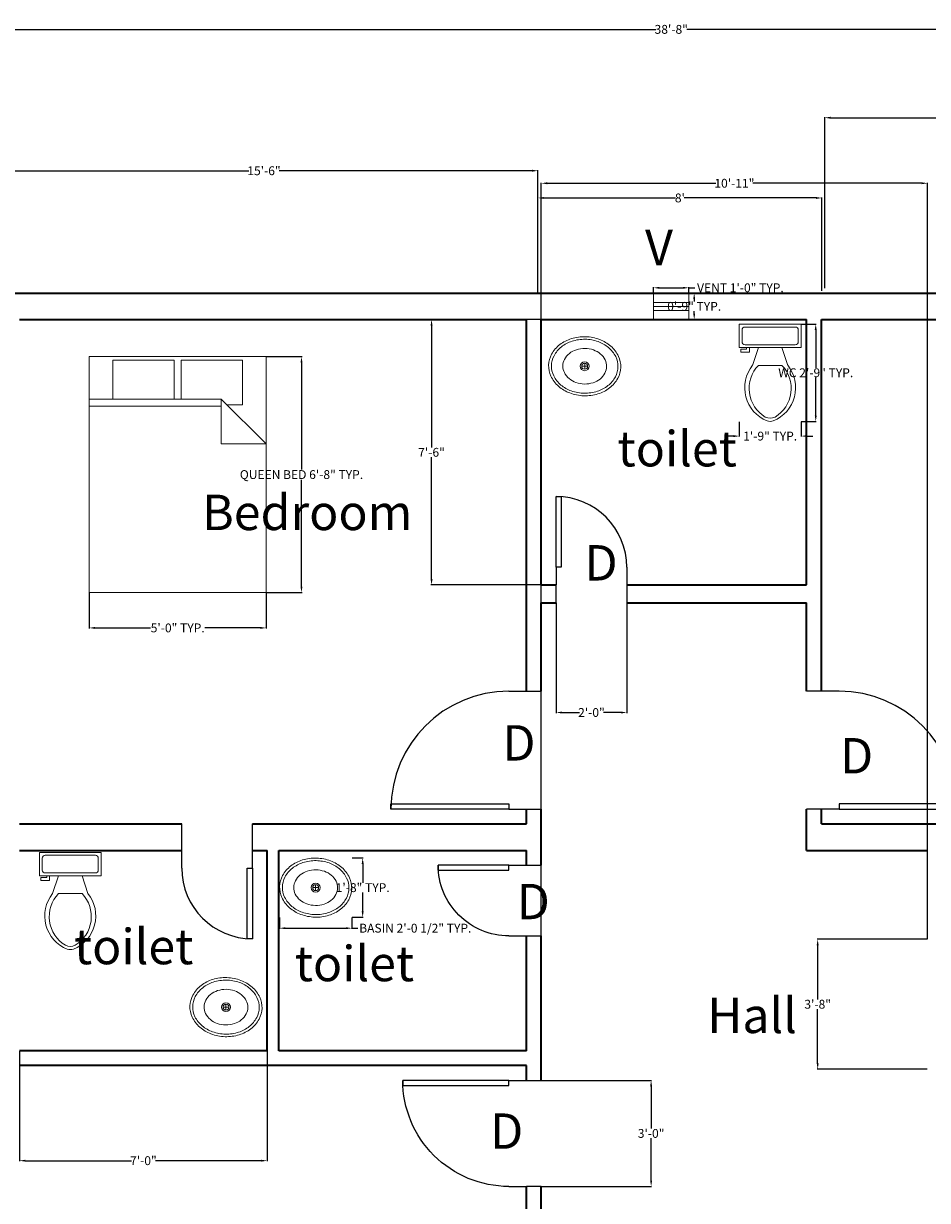
# Model space of a CAD drawing. Units: inches. Extents: x 751 to 1500, y 610 to 1297.
# Tile 3 of 4: x 1001 to 1308, y 898 to 1297. Entities that reach past the tile are written whole.
import ezdxf

# ---------------------------------------------------------------- set-up
doc = ezdxf.new("R2010")
doc.units = ezdxf.units.IN
doc.header["$MEASUREMENT"] = 0
doc.layers.get('0').update_dxf_attribs({"color": 1})
for name, color, linetype, lineweight in [('A-ANNO-DIMS', 5, 'Continuous', 18), ('A-ANNO-TEXT', 7, 'Continuous', 18), ('A-AREA-IDEN', 7, 'Continuous', 25), ('A-FLOR-FIXT', 9, 'Continuous', 18), ('A-FURN', 8, 'Continuous', 18), ('door', 2, 'Continuous', 25), ('wall', 6, 'Continuous', 35), ('windows', 70, 'Continuous', 18)]:
    doc.layers.add(name, color=color, linetype=linetype, lineweight=lineweight)
doc.styles.get("Standard").update_dxf_attribs({"font": 'arial.ttf'})
doc.dimstyles.get("Standard").update_dxf_attribs({"dimtxt": 3, "dimasz": 2, "dimexe": 0.18, "dimexo": 0.0625, "dimgap": 0.09, "dimtad": 0, "dimtih": 1, "dimtoh": 1, "dimdec": 0, "dimzin": 0, "dimdsep": 46, "dimlunit": 3, "dimtxsty": 'Standard', "dimcen": 0.09, "dimadec": 0, "dimazin": 0, "dimtfac": 1, "dimtdec": 0, "dimtofl": 0, "dimtmove": 0, "dimatfit": 3, "dimfxl": 1, "dimtolj": 1, "dimtzin": 0, "dimarcsym": 0})

# ---------------------------------------------------------------- blocks, each defined once
blk = doc.blocks.new('*U2')
for p, q in [((0, 0), (0, -6)), ((40, 0), (40, -6))]:
    blk.add_line(p, q)
blk.add_lwpolyline([(0, 0), (0, 40), (1.75, 40), (1.75, 0)], close=True)
blk.add_arc((0, 0), 40, 0, 90)
blk = doc.blocks.new('*U3')
for p, q in [((0, 0), (0, 6)), ((40, 0), (40, 6))]:
    blk.add_line(p, q)
blk.add_lwpolyline([(0, 0), (0, -40), (1.75, -40), (1.75, 0)], close=True)
blk.add_arc((0, 0), 40, 270, 360)
blk = doc.blocks.new('*U4')
for p, q in [((0, 0), (0, -6)), ((24, 0), (24, -6))]:
    blk.add_line(p, q)
blk.add_lwpolyline([(0, 0), (0, 24), (1.75, 24), (1.75, 0)], close=True)
blk.add_arc((0, 0), 24, 0, 90)
blk = doc.blocks.new('*U7')
for p, q in [((0, 0), (0, -6)), ((36, 0), (36, -6))]:
    blk.add_line(p, q)
blk.add_lwpolyline([(0, 0), (0, 36), (1.75, 36), (1.75, 0)], close=True)
blk.add_arc((0, 0), 36, 0, 90)
blk = doc.blocks.new('*D8')
at = {"layer": 'A-ANNO-DIMS', "color": 0, "lineweight": -2, "transparency": 16777216}
for p, q in [((989.16, 1207.18), (989.16, 1295.32)), ((991.16, 1295.14), (1215.8, 1295.14)), ((1450.93, 1295.14), (1226.29, 1295.14)), ((1452.93, 1205.96), (1452.93, 1295.32))]:
    blk.add_line(p, q, dxfattribs=at)
at = {"layer": 'A-ANNO-DIMS', "color": 0, "transparency": 16777216}
for points in [[(991.16, 1295.48), (991.16, 1294.81), (989.16, 1295.14)], [(1450.93, 1295.48), (1450.93, 1294.81), (1452.93, 1295.14)]]:
    blk.add_solid(points, dxfattribs=at)
at = {"layer": 'Defpoints', "color": 0, "transparency": 16777216}
for p in [(1452.93, 1295.14), (989.16, 1207.12), (1452.93, 1205.9)]:
    blk.add_point(p, dxfattribs=at)
at = {"layer": 'A-ANNO-DIMS', "color": 0, "transparency": 16777216, "insert": (1221.05, 1295.14), "char_height": 3, "attachment_point": 5}
blk.add_mtext('\\A1;38\'-8"', dxfattribs=at)
blk = doc.blocks.new('*D9')
at = {"layer": 'A-ANNO-DIMS', "color": 0, "lineweight": -2, "transparency": 16777216}
for p, q in [((989.97, 1205.95), (989.97, 1247.37)), ((991.97, 1247.19), (1077.79, 1247.19)), ((1173.82, 1247.19), (1088, 1247.19)), ((1175.82, 1205.95), (1175.82, 1247.37))]:
    blk.add_line(p, q, dxfattribs=at)
at = {"layer": 'A-ANNO-DIMS', "color": 0, "transparency": 16777216}
for points in [[(991.97, 1247.53), (991.97, 1246.86), (989.97, 1247.19)], [(1173.82, 1247.53), (1173.82, 1246.86), (1175.82, 1247.19)]]:
    blk.add_solid(points, dxfattribs=at)
at = {"layer": 'Defpoints', "color": 0, "transparency": 16777216}
for p in [(1175.82, 1247.19), (989.97, 1205.88), (1175.82, 1205.88)]:
    blk.add_point(p, dxfattribs=at)
at = {"layer": 'A-ANNO-DIMS', "color": 0, "transparency": 16777216, "insert": (1082.89, 1247.19), "char_height": 3, "attachment_point": 5}
blk.add_mtext('\\A1;15\'-6"', dxfattribs=at)
blk = doc.blocks.new('*D10')
at = {"layer": 'A-ANNO-DIMS', "color": 0, "lineweight": -2, "transparency": 16777216}
for p, q in [((1175.82, 1206.43), (1175.82, 1238.14)), ((1177.82, 1237.96), (1222.52, 1237.96)), ((1270.16, 1237.96), (1225.46, 1237.96)), ((1272.16, 1206.43), (1272.16, 1238.14))]:
    blk.add_line(p, q, dxfattribs=at)
at = {"layer": 'A-ANNO-DIMS', "color": 0, "transparency": 16777216}
for points in [[(1177.82, 1238.29), (1177.82, 1237.63), (1175.82, 1237.96)], [(1270.16, 1238.29), (1270.16, 1237.63), (1272.16, 1237.96)]]:
    blk.add_solid(points, dxfattribs=at)
at = {"layer": 'Defpoints', "color": 0, "transparency": 16777216}
for p in [(1272.16, 1237.96), (1175.82, 1206.37), (1272.16, 1206.37)]:
    blk.add_point(p, dxfattribs=at)
at = {"layer": 'A-ANNO-DIMS', "color": 0, "transparency": 16777216, "insert": (1223.99, 1237.96), "char_height": 3, "attachment_point": 5}
blk.add_mtext("\\A1;8'", dxfattribs=at)
blk = doc.blocks.new('*D11')
at = {"layer": 'A-ANNO-DIMS', "color": 0, "lineweight": -2, "transparency": 16777216}
for p, q in [((1273.13, 1207.41), (1273.13, 1265.35)), ((1452.66, 1205.46), (1452.66, 1265.35)), ((1275.13, 1265.17), (1360.4, 1265.17)), ((1450.66, 1265.17), (1365.39, 1265.17))]:
    blk.add_line(p, q, dxfattribs=at)
at = {"layer": 'A-ANNO-DIMS', "color": 0, "transparency": 16777216}
for points in [[(1275.13, 1265.51), (1275.13, 1264.84), (1273.13, 1265.17)], [(1450.66, 1265.51), (1450.66, 1264.84), (1452.66, 1265.17)]]:
    blk.add_solid(points, dxfattribs=at)
at = {"layer": 'Defpoints', "color": 0, "transparency": 16777216}
for p in [(1452.66, 1265.17), (1273.13, 1207.34), (1452.66, 1205.4)]:
    blk.add_point(p, dxfattribs=at)
at = {"layer": 'A-ANNO-DIMS', "color": 0, "transparency": 16777216, "insert": (1362.9, 1265.17), "char_height": 3, "attachment_point": 5}
blk.add_mtext("\\A1;15'", dxfattribs=at)
blk = doc.blocks.new('Bed - Queen')
for p, q in [((0, -80.00003), (0, 0)), ((0, 0), (59.99999, 0)), ((59.99999, 0), (59.99999, -80.00003)), ((7.99999, -1.2), (28.79998, -1.2)), ((7.99999, -14.4), (7.99999, -1.2)), ((28.79998, -1.2), (28.79998, -14.4)), ((31.19999, -1.2), (51.99999, -1.2)), ((31.19999, -14.4), (31.19999, -1.2)), ((51.99999, -1.2), (51.99999, -16.4)), ((0, -14.4), (44.8, -14.4)), ((59.99999, -29.6), (44.8, -14.4)), ((44.8, -14.4), (44.8, -29.6)), ((44.8, -16.8), (0, -16.8)), ((51.99999, -16.4), (46.79936, -16.4)), ((44.8, -29.6), (59.99999, -29.6)), ((59.99999, -80.00003), (0, -80.00003))]:
    blk.add_line(p, q)
blk = doc.blocks.new('Sink - Oval top')
for p, q in [((-1, 0), (1, 0)), ((0, 1), (0, -1))]:
    blk.add_line(p, q)
for points in [[(-12.23, 0.39, 0.117634), (-11.46, -3.36, 0.104469), (-8.88, -6.8, 0.090016), (-5.08, -9.07, 0.08192), (-0.32, -10.02, 0.08192), (4.49, -9.38, 0.090016), (8.42, -7.36, 0.104469), (11.22, -4.09, 0.117634), (12.23, -0.39, 0.117634), (11.46, 3.36, 0.104469), (8.88, 6.8, 0.090016), (5.08, 9.07, 0.08192), (0.32, 10.02, 0.08192), (-4.49, 9.38, 0.090016), (-8.42, 7.36, 0.104469), (-11.22, 4.09, 0.117634)], [(-11.29, 0.16, 0.118622), (-10.52, -3.25, 0.104678), (-8.07, -6.36, 0.089562), (-4.54, -8.37, 0.081185), (-0.13, -9.15, 0.081185), (4.3, -8.49, 0.089562), (7.89, -6.58, 0.104678), (10.42, -3.55, 0.118622), (11.29, -0.16, 0.118622), (10.52, 3.25, 0.104678), (8.07, 6.36, 0.089562), (4.54, 8.37, 0.081185), (0.13, 9.15, 0.081185), (-4.3, 8.49, 0.089562), (-7.89, 6.58, 0.104678), (-10.42, 3.55, 0.118622)], [(-7.42, 0.08, 0.118283), (-6.91, -2.17, 0.104607), (-5.29, -4.21, 0.089718), (-2.97, -5.53, 0.081436), (-0.07, -6.04, 0.081436), (2.84, -5.59, 0.089718), (5.2, -4.33, 0.104607), (6.86, -2.32, 0.118283), (7.42, -0.08, 0.118283), (6.91, 2.17, 0.104607), (5.29, 4.21, 0.089718), (2.97, 5.53, 0.081436), (0.07, 6.04, 0.081436), (-2.84, 5.59, 0.089718), (-5.2, 4.33, 0.104607), (-6.86, 2.32, 0.118283)]]:
    blk.add_lwpolyline(points, format="xyb", close=True)
for radius in [1.5, 1]:
    blk.add_circle((0, 0), radius)
blk = doc.blocks.new('Toilet - top')
for p, q in [((9.5, -6), (9.5, -2)), ((-10, -8.5), (-8, -8.5)), ((-10, -9.5), (-10, -8.5)), ((-7, -9.5), (-10, -9.5)), ((-8, -8.5), (-8, -8)), ((-7, -8), (-7, -9.5)), ((-4, -8), (-6, -14)), ((4, -8), (6, -14)), ((4, -14), (-4, -14))]:
    blk.add_line(p, q)
blk.add_lwpolyline([(10.5, -8), (10.5, 0), (-10.5, 0), (-10.5, -8)], close=True)
for points in [[(-9.5, -2), (-9.5, -6)], [(8.5, -1), (-8.5, -1)], [(-8.5, -7), (8.5, -7)]]:
    blk.add_lwpolyline(points)
for centre, radius, start, end in [((-8.62, -1.88), 0.884, 81.8699, 188.1301), ((8.62, -1.88), 0.884, 351.8699, 98.1301), ((-8.62, -6.12), 0.884, 171.8699, 278.1301), ((8.62, -6.12), 0.884, 261.8699, 8.1301), ((3.52, -21.58), 12.17, 141.4691, 247.9714), ((4.2, -21.82), 11.33, 136.3677, 238.9468), ((-3.52, -21.58), 12.17, 292.0284, 38.5307), ((-4.2, -21.82), 11.33, 301.053, 43.6321), ((0, -27.88), 4, 245.7318, 294.2682), ((0, -29), 4, 254.8605, 285.1395)]:
    blk.add_arc(centre, radius, start, end)
blk = doc.blocks.new('VENT-12IN-PLAN')
for p, q in [((3.14, 12), (3.14, 0)), ((4.5, 12), (4.5, 0)), ((5.86, 12), (5.86, 0))]:
    blk.add_line(p, q)
blk.add_lwpolyline([(0, 0), (9, 0), (9, 12), (0, 12)], close=True)
blk = doc.blocks.new('*D31')
at = {"layer": 'A-ANNO-DIMS', "color": 0, "lineweight": -2, "transparency": 16777216}
for p, q in [((1215.04, 1205.75), (1215.04, 1207.67)), ((1217.04, 1207.49), (1225.04, 1207.49)), ((1227.04, 1205.75), (1227.04, 1207.67)), ((1227.04, 1207.49), (1229.04, 1207.49))]:
    blk.add_line(p, q, dxfattribs=at)
at = {"layer": 'A-ANNO-DIMS', "color": 0, "transparency": 16777216}
for points in [[(1217.04, 1207.82), (1217.04, 1207.16), (1215.04, 1207.49)], [(1225.04, 1207.82), (1225.04, 1207.16), (1227.04, 1207.49)]]:
    blk.add_solid(points, dxfattribs=at)
at = {"layer": 'Defpoints', "color": 0, "transparency": 16777216}
for p in [(1215.04, 1205.69), (1227.04, 1207.49), (1227.04, 1205.69)]:
    blk.add_point(p, dxfattribs=at)
at = {"layer": 'A-ANNO-DIMS', "color": 0, "transparency": 16777216, "insert": (1244.52, 1207.49), "char_height": 3, "attachment_point": 5}
blk.add_mtext('\\A1;VENT 1\'-0" TYP.', dxfattribs=at)
blk = doc.blocks.new('*D32')
at = {"layer": 'A-ANNO-DIMS', "color": 0, "lineweight": -2, "transparency": 16777216}
for p, q in [((1227.1, 1205.69), (1229.02, 1205.69)), ((1228.84, 1203.69), (1228.84, 1202.81)), ((1228.84, 1198.69), (1228.84, 1199.57)), ((1227.1, 1196.69), (1229.02, 1196.69))]:
    blk.add_line(p, q, dxfattribs=at)
at = {"layer": 'A-ANNO-DIMS', "color": 0, "transparency": 16777216}
for points in [[(1228.51, 1203.69), (1229.17, 1203.69), (1228.84, 1205.69)], [(1228.51, 1198.69), (1229.17, 1198.69), (1228.84, 1196.69)]]:
    blk.add_solid(points, dxfattribs=at)
at = {"layer": 'Defpoints', "color": 0, "transparency": 16777216}
for p in [(1227.04, 1205.69), (1227.04, 1196.69), (1228.84, 1196.69)]:
    blk.add_point(p, dxfattribs=at)
at = {"layer": 'A-ANNO-DIMS', "color": 0, "transparency": 16777216, "insert": (1228.84, 1201.19), "char_height": 3, "attachment_point": 5}
blk.add_mtext('\\A1;0\'-9" TYP.', dxfattribs=at)
blk = doc.blocks.new('*D33')
at = {"layer": 'A-ANNO-DIMS', "color": 0, "lineweight": -2, "transparency": 16777216}
for p, q in [((1083.67, 1184.14), (1095.79, 1184.14)), ((1095.61, 1182.14), (1095.61, 1145.87)), ((1095.61, 1106.14), (1095.61, 1142.4)), ((1083.67, 1104.14), (1095.79, 1104.14))]:
    blk.add_line(p, q, dxfattribs=at)
at = {"layer": 'A-ANNO-DIMS', "color": 0, "transparency": 16777216}
for points in [[(1095.28, 1182.14), (1095.95, 1182.14), (1095.61, 1184.14)], [(1095.28, 1106.14), (1095.95, 1106.14), (1095.61, 1104.14)]]:
    blk.add_solid(points, dxfattribs=at)
at = {"layer": 'Defpoints', "color": 0, "transparency": 16777216}
for p in [(1083.61, 1184.14), (1095.61, 1184.14), (1083.61, 1104.14)]:
    blk.add_point(p, dxfattribs=at)
at = {"layer": 'A-ANNO-DIMS', "color": 0, "transparency": 16777216, "insert": (1095.61, 1144.14), "char_height": 3, "attachment_point": 5}
blk.add_mtext('\\A1;QUEEN BED 6\'-8" TYP.', dxfattribs=at)
blk = doc.blocks.new('*D34')
at = {"layer": 'A-ANNO-DIMS', "color": 0, "lineweight": -2, "transparency": 16777216}
for p, q in [((1023.61, 1104.07), (1023.61, 1091.96)), ((1083.61, 1104.07), (1083.61, 1091.96)), ((1025.61, 1092.14), (1044.38, 1092.14)), ((1081.61, 1092.14), (1062.85, 1092.14))]:
    blk.add_line(p, q, dxfattribs=at)
at = {"layer": 'A-ANNO-DIMS', "color": 0, "transparency": 16777216}
for points in [[(1025.61, 1092.47), (1025.61, 1091.8), (1023.61, 1092.14)], [(1081.61, 1092.47), (1081.61, 1091.8), (1083.61, 1092.14)]]:
    blk.add_solid(points, dxfattribs=at)
at = {"layer": 'Defpoints', "color": 0, "transparency": 16777216}
for p in [(1023.61, 1104.14), (1083.61, 1104.14), (1083.61, 1092.14)]:
    blk.add_point(p, dxfattribs=at)
at = {"layer": 'A-ANNO-DIMS', "color": 0, "transparency": 16777216, "insert": (1053.61, 1092.14), "char_height": 3, "attachment_point": 5}
blk.add_mtext('\\A1;5\'-0" TYP.', dxfattribs=at)
blk = doc.blocks.new('*D35')
at = {"layer": 'A-ANNO-DIMS', "color": 0, "lineweight": -2, "transparency": 16777216}
for p, q in [((1088.14, 993.92), (1088.14, 990.12)), ((1112.69, 993.92), (1112.69, 990.12)), ((1090.14, 990.3), (1110.69, 990.3)), ((1112.69, 990.3), (1114.69, 990.3))]:
    blk.add_line(p, q, dxfattribs=at)
at = {"layer": 'A-ANNO-DIMS', "color": 0, "transparency": 16777216}
for points in [[(1090.14, 990.63), (1090.14, 989.96), (1088.14, 990.3)], [(1110.69, 990.63), (1110.69, 989.96), (1112.69, 990.3)]]:
    blk.add_solid(points, dxfattribs=at)
at = {"layer": 'Defpoints', "color": 0, "transparency": 16777216}
for p in [(1088.14, 993.98), (1112.69, 993.98), (1112.69, 990.3)]:
    blk.add_point(p, dxfattribs=at)
at = {"layer": 'A-ANNO-DIMS', "color": 0, "transparency": 16777216, "insert": (1134.22, 990.3), "char_height": 3, "attachment_point": 5}
blk.add_mtext('\\A1;BASIN 2\'-0 1/2" TYP.', dxfattribs=at)
blk = doc.blocks.new('*D36')
at = {"layer": 'A-ANNO-DIMS', "color": 0, "lineweight": -2, "transparency": 16777216}
for p, q in [((1112.75, 1014.12), (1116.55, 1014.12)), ((1116.37, 1012.12), (1116.37, 1005.67)), ((1116.37, 995.98), (1116.37, 1002.43)), ((1112.75, 993.98), (1116.55, 993.98))]:
    blk.add_line(p, q, dxfattribs=at)
at = {"layer": 'A-ANNO-DIMS', "color": 0, "transparency": 16777216}
for points in [[(1116.04, 1012.12), (1116.71, 1012.12), (1116.37, 1014.12)], [(1116.04, 995.98), (1116.71, 995.98), (1116.37, 993.98)]]:
    blk.add_solid(points, dxfattribs=at)
at = {"layer": 'Defpoints', "color": 0, "transparency": 16777216}
for p in [(1112.69, 1014.12), (1116.37, 1014.12), (1112.69, 993.98)]:
    blk.add_point(p, dxfattribs=at)
at = {"layer": 'A-ANNO-DIMS', "color": 0, "transparency": 16777216, "insert": (1116.37, 1004.05), "char_height": 3, "attachment_point": 5}
blk.add_mtext('\\A1;1\'-8" TYP.', dxfattribs=at)
blk = doc.blocks.new('*D37')
at = {"layer": 'A-ANNO-DIMS', "color": 0, "lineweight": -2, "transparency": 16777216}
for p, q in [((1265.18, 1195.19), (1270.26, 1195.19)), ((1270.08, 1193.19), (1270.08, 1180.31)), ((1270.08, 1164.14), (1270.08, 1177.03)), ((1265.18, 1162.14), (1270.26, 1162.14))]:
    blk.add_line(p, q, dxfattribs=at)
at = {"layer": 'A-ANNO-DIMS', "color": 0, "transparency": 16777216}
for points in [[(1269.74, 1193.19), (1270.41, 1193.19), (1270.08, 1195.19)], [(1269.74, 1164.14), (1270.41, 1164.14), (1270.08, 1162.14)]]:
    blk.add_solid(points, dxfattribs=at)
at = {"layer": 'Defpoints', "color": 0, "transparency": 16777216}
for p in [(1265.12, 1195.19), (1270.08, 1195.19), (1265.12, 1162.14)]:
    blk.add_point(p, dxfattribs=at)
at = {"layer": 'A-ANNO-DIMS', "color": 0, "transparency": 16777216, "insert": (1270.08, 1178.67), "char_height": 3, "attachment_point": 5}
blk.add_mtext('\\A1;WC 2\'-9" TYP.', dxfattribs=at)
blk = doc.blocks.new('*D38')
at = {"layer": 'A-ANNO-DIMS', "color": 0, "lineweight": -2, "transparency": 16777216}
for p, q in [((1244.12, 1162.08), (1244.12, 1157.01)), ((1265.12, 1162.08), (1265.12, 1157.01)), ((1242.12, 1157.19), (1240.12, 1157.19)), ((1267.12, 1157.19), (1269.12, 1157.19))]:
    blk.add_line(p, q, dxfattribs=at)
at = {"layer": 'A-ANNO-DIMS', "color": 0, "transparency": 16777216}
for points in [[(1242.12, 1157.52), (1242.12, 1156.85), (1244.12, 1157.19)], [(1267.12, 1157.52), (1267.12, 1156.85), (1265.12, 1157.19)]]:
    blk.add_solid(points, dxfattribs=at)
at = {"layer": 'Defpoints', "color": 0, "transparency": 16777216}
for p in [(1244.12, 1162.14), (1265.12, 1162.14), (1265.12, 1157.19)]:
    blk.add_point(p, dxfattribs=at)
at = {"layer": 'A-ANNO-DIMS', "color": 0, "transparency": 16777216, "insert": (1254.62, 1157.19), "char_height": 3, "attachment_point": 5}
blk.add_mtext('\\A1;1\'-9" TYP.', dxfattribs=at)
blk = doc.blocks.new('*D54')
at = {"layer": 'A-ANNO-DIMS', "color": 0, "lineweight": -2, "transparency": 16777216}
for p, q in [((999.98, 948.63), (999.98, 911.26)), ((1083.98, 948.63), (1083.98, 911.26)), ((1001.98, 911.44), (1037.92, 911.44)), ((1081.98, 911.44), (1046.05, 911.44))]:
    blk.add_line(p, q, dxfattribs=at)
at = {"layer": 'A-ANNO-DIMS', "color": 0, "transparency": 16777216}
for points in [[(1001.98, 911.77), (1001.98, 911.11), (999.98, 911.44)], [(1081.98, 911.77), (1081.98, 911.11), (1083.98, 911.44)]]:
    blk.add_solid(points, dxfattribs=at)
at = {"layer": 'Defpoints', "color": 0, "transparency": 16777216}
for p in [(999.98, 948.69), (1083.98, 948.69), (999.98, 911.44)]:
    blk.add_point(p, dxfattribs=at)
at = {"layer": 'A-ANNO-DIMS', "color": 0, "transparency": 16777216, "insert": (1041.98, 911.44), "char_height": 3, "attachment_point": 5}
blk.add_mtext('\\A1;7\'-0"', dxfattribs=at)
blk = doc.blocks.new('*D56')
at = {"layer": 'A-ANNO-DIMS', "color": 0, "lineweight": -2, "transparency": 16777216}
for p, q in [((1176.92, 1196.69), (1139.55, 1196.69)), ((1139.73, 1194.69), (1139.73, 1153.31)), ((1139.73, 1108.69), (1139.73, 1150.07)), ((1176.92, 1106.69), (1139.55, 1106.69))]:
    blk.add_line(p, q, dxfattribs=at)
at = {"layer": 'A-ANNO-DIMS', "color": 0, "transparency": 16777216}
for points in [[(1139.4, 1194.69), (1140.07, 1194.69), (1139.73, 1196.69)], [(1139.4, 1108.69), (1140.07, 1108.69), (1139.73, 1106.69)]]:
    blk.add_solid(points, dxfattribs=at)
at = {"layer": 'Defpoints', "color": 0, "transparency": 16777216}
for p in [(1139.73, 1196.69), (1176.98, 1196.69), (1176.98, 1106.69)]:
    blk.add_point(p, dxfattribs=at)
at = {"layer": 'A-ANNO-DIMS', "color": 0, "transparency": 16777216, "insert": (1139.73, 1151.69), "char_height": 3, "attachment_point": 5}
blk.add_mtext('\\A1;7\'-6"', dxfattribs=at)
blk = doc.blocks.new('*D58')
at = {"layer": 'A-ANNO-DIMS', "color": 0, "lineweight": -2, "transparency": 16777216}
for p, q in [((1177.04, 938.69), (1214.41, 938.69)), ((1214.23, 936.69), (1214.23, 922.31)), ((1214.23, 904.69), (1214.23, 919.07)), ((1177.04, 902.69), (1214.41, 902.69))]:
    blk.add_line(p, q, dxfattribs=at)
at = {"layer": 'A-ANNO-DIMS', "color": 0, "transparency": 16777216}
for points in [[(1213.9, 936.69), (1214.57, 936.69), (1214.23, 938.69)], [(1213.9, 904.69), (1214.57, 904.69), (1214.23, 902.69)]]:
    blk.add_solid(points, dxfattribs=at)
at = {"layer": 'Defpoints', "color": 0, "transparency": 16777216}
for p in [(1176.98, 938.69), (1176.98, 902.69), (1214.23, 902.69)]:
    blk.add_point(p, dxfattribs=at)
at = {"layer": 'A-ANNO-DIMS', "color": 0, "transparency": 16777216, "insert": (1214.23, 920.69), "char_height": 3, "attachment_point": 5}
blk.add_mtext('\\A1;3\'-0"', dxfattribs=at)
blk = doc.blocks.new('*D59')
at = {"layer": 'A-ANNO-DIMS', "color": 0, "lineweight": -2, "transparency": 16777216}
for p, q in [((1181.98, 1100.63), (1181.98, 1063.26)), ((1205.98, 1100.63), (1205.98, 1063.26)), ((1183.98, 1063.44), (1189.88, 1063.44)), ((1203.98, 1063.44), (1198.09, 1063.44))]:
    blk.add_line(p, q, dxfattribs=at)
at = {"layer": 'A-ANNO-DIMS', "color": 0, "transparency": 16777216}
for points in [[(1183.98, 1063.77), (1183.98, 1063.11), (1181.98, 1063.44)], [(1203.98, 1063.77), (1203.98, 1063.11), (1205.98, 1063.44)]]:
    blk.add_solid(points, dxfattribs=at)
at = {"layer": 'Defpoints', "color": 0, "transparency": 16777216}
for p in [(1181.98, 1100.69), (1205.98, 1100.69), (1181.98, 1063.44)]:
    blk.add_point(p, dxfattribs=at)
at = {"layer": 'A-ANNO-DIMS', "color": 0, "transparency": 16777216, "insert": (1193.98, 1063.44), "char_height": 3, "attachment_point": 5}
blk.add_mtext('\\A1;2\'-0"', dxfattribs=at)
blk = doc.blocks.new('*D62')
at = {"layer": 'A-ANNO-DIMS', "color": 0, "lineweight": -2, "transparency": 16777216}
for p, q in [((1176.98, 987.75), (1176.98, 1243.12)), ((1178.98, 1242.94), (1236.22, 1242.94)), ((1305.98, 1242.94), (1248.75, 1242.94)), ((1307.98, 986.59), (1307.98, 1243.12))]:
    blk.add_line(p, q, dxfattribs=at)
at = {"layer": 'A-ANNO-DIMS', "color": 0, "transparency": 16777216}
for points in [[(1178.98, 1243.27), (1178.98, 1242.61), (1176.98, 1242.94)], [(1305.98, 1243.27), (1305.98, 1242.61), (1307.98, 1242.94)]]:
    blk.add_solid(points, dxfattribs=at)
at = {"layer": 'Defpoints', "color": 0, "transparency": 16777216}
for p in [(1307.98, 1242.94), (1176.98, 987.69), (1307.98, 986.52)]:
    blk.add_point(p, dxfattribs=at)
at = {"layer": 'A-ANNO-DIMS', "color": 0, "transparency": 16777216, "insert": (1242.48, 1242.94), "char_height": 3, "attachment_point": 5}
blk.add_mtext('\\A1;10\'-11"', dxfattribs=at)
blk = doc.blocks.new('*D66')
at = {"layer": 'A-ANNO-DIMS', "color": 0, "lineweight": -2, "transparency": 16777216}
for p, q in [((1307.92, 986.52), (1270.55, 986.52)), ((1270.73, 984.52), (1270.73, 966.12)), ((1270.73, 944.48), (1270.73, 962.88)), ((1307.92, 942.48), (1270.55, 942.48))]:
    blk.add_line(p, q, dxfattribs=at)
at = {"layer": 'A-ANNO-DIMS', "color": 0, "transparency": 16777216}
for points in [[(1270.4, 984.52), (1271.07, 984.52), (1270.73, 986.52)], [(1270.4, 944.48), (1271.07, 944.48), (1270.73, 942.48)]]:
    blk.add_solid(points, dxfattribs=at)
at = {"layer": 'Defpoints', "color": 0, "transparency": 16777216}
for p in [(1270.73, 986.52), (1307.98, 986.52), (1307.98, 942.48)]:
    blk.add_point(p, dxfattribs=at)
at = {"layer": 'A-ANNO-DIMS', "color": 0, "transparency": 16777216, "insert": (1270.73, 964.5), "char_height": 3, "attachment_point": 5}
blk.add_mtext('\\A1;3\'-8"', dxfattribs=at)

msp = doc.modelspace()

# ---------------------------------------------------------------- linework, layer by layer
at = {"layer": 'door'}
for p, q in [((1181.98, 1100.69), (1181.98, 1106.69)), ((1205.98, 1106.69), (1205.98, 1100.69)), ((1171.98, 1070.69), (1176.98, 1070.69)), ((1271.98, 1070.69), (1266.98, 1070.69)), ((1171.98, 1030.69), (1176.98, 1030.69)), ((1271.98, 1030.69), (1266.98, 1030.69)), ((1054.98, 1016.69), (1054.98, 1025.69)), ((1078.98, 1016.69), (1078.98, 1025.69)), ((1171.98, 1011.69), (1176.98, 1011.69)), ((1171.98, 987.69), (1176.98, 987.69)), ((1171.98, 938.69), (1176.98, 938.69)), ((1176.98, 902.69), (1171.98, 902.69))]:
    msp.add_line(p, q, dxfattribs=at)
at = {"layer": 'wall'}
for p, q in [((990.98, 1205.69), (1296.98, 1205.69)), ((1296.98, 1205.69), (1453.98, 1205.69)), ((999.98, 1196.69), (1171.98, 1196.69)), ((1171.98, 1070.69), (1171.98, 1196.69)), ((1176.98, 1196.69), (1266.98, 1196.69)), ((1176.98, 1106.69), (1176.98, 1196.69)), ((1266.98, 1106.69), (1266.98, 1196.69)), ((1271.98, 1196.69), (1296.98, 1196.69)), ((1271.98, 1070.69), (1271.98, 1196.69)), ((1296.98, 1196.69), (1444.98, 1196.69)), ((1176.98, 1106.69), (1181.98, 1106.69)), ((1205.98, 1106.69), (1266.98, 1106.69)), ((1176.98, 1070.69), (1176.98, 1100.69)), ((1176.98, 1100.69), (1181.98, 1100.69)), ((1205.98, 1100.69), (1266.98, 1100.69)), ((1266.98, 1070.69), (1266.98, 1100.69)), ((1171.98, 1025.69), (1171.98, 1030.69)), ((1176.98, 1011.69), (1176.98, 1030.69)), ((1266.98, 1016.69), (1266.98, 1030.69)), ((1271.98, 1025.69), (1271.98, 1030.69)), ((999.98, 1025.69), (1054.98, 1025.69)), ((1078.98, 1025.69), (1171.98, 1025.69)), ((1271.98, 1025.69), (1444.98, 1025.69)), ((999.98, 1016.69), (1054.98, 1016.69)), ((1078.98, 1016.69), (1083.98, 1016.69)), ((1083.98, 986.69), (1083.98, 1016.69)), ((1087.98, 948.69), (1087.98, 1016.69)), ((1087.98, 1016.69), (1171.98, 1016.69)), ((1171.98, 1011.69), (1171.98, 1016.69)), ((1266.98, 1016.69), (1307.98, 1016.69)), ((1083.98, 948.69), (1083.98, 986.69)), ((1171.98, 948.69), (1171.98, 987.69)), ((1176.98, 938.69), (1176.98, 987.69)), ((1083.98, 948.69), (999.98, 948.69)), ((1171.98, 948.69), (1087.98, 948.69)), ((1171.98, 943.69), (999.98, 943.69)), ((1171.98, 938.69), (1171.98, 943.69)), ((1171.98, 787.69), (1171.98, 902.69)), ((1176.98, 787.69), (1176.98, 902.69))]:
    msp.add_line(p, q, dxfattribs=at)

# ---------------------------------------------------------------- block references
at = {"layer": 'A-FLOR-FIXT'}
for name, p in [('Toilet - top', (1254.62, 1195.19)), ('Sink - Oval top', (1191.7, 1180.88)), ('Toilet - top', (1017.18, 1016.02)), ('Sink - Oval top', (1100.42, 1004.05)), ('Sink - Oval top', (1069.99, 963.52))]:
    msp.add_blockref(name, p, dxfattribs=at)
at = {"layer": 'A-FURN'}
msp.add_blockref('Bed - Queen', (1023.61, 1184.14), dxfattribs=at)
at = {"layer": 'door'}
msp.add_blockref('*U4', (1181.98, 1112.69), dxfattribs=at)
for name, p, rotation in [('*U2', (1165.98, 1030.69), 90), ('*U3', (1277.98, 1030.69), 90), ('*U4', (1078.98, 1010.69), 180)]:
    msp.add_blockref(name, p, dxfattribs=dict(at, rotation=rotation))
at = {"layer": 'door', "xscale": -1, "rotation": 89.99999999999737}
for name, p in [('*U4', (1165.98, 1011.69)), ('*U7', (1165.98, 938.69))]:
    msp.add_blockref(name, p, dxfattribs=at)
at = {"layer": 'windows', "rotation": 269.9999999999972}
msp.add_blockref('VENT-12IN-PLAN', (1215.04, 1205.69), dxfattribs=at)

# ---------------------------------------------------------------- texts
at = {"layer": 'A-ANNO-TEXT', "char_height": 12, "attachment_point": 1}
for s, width, heights, insert in [('V', 67.5718, [0], (1212.19, 1227.16)), ('D', 17.3049, [0.2], (1191.62, 1120.21)), ('D', 17.3049, [0.2], (1191.62, 1120.21)), ('D', 17.3049, [0.2], (1163.75, 1059.14)), ('D', 17.3049, [0.2], (1278.31, 1054.78)), ('D', 17.3049, [0.2], (1168.61, 1005.32)), ('D', 17.3049, [0.2], (1159.59, 927.48))]:
    msp.add_mtext_dynamic_manual_height_columns(s, width=width, gutter_width=1, heights=heights, dxfattribs=dict(at, insert=insert))
at = {"layer": 'A-AREA-IDEN', "char_height": 12, "attachment_point": 1}
for s, width, insert in [('toilet', 75.006, (1202.83, 1158.91)), ('Bedroom', 61.9104, (1061.89, 1137.31)), ('toilet', 75.006, (1018.42, 990.07)), ('toilet', 75.006, (1093.33, 984.31)), ('Hall', 38.6311, (1233.26, 966.72))]:
    msp.add_mtext_dynamic_manual_height_columns(s, width=width, gutter_width=1, heights=[0], dxfattribs=dict(at, insert=insert))

# ---------------------------------------------------------------- dimensions: what is measured, and where the dimension line sits
at = {"layer": 'A-ANNO-DIMS'}
for base, p1, p2, override, picture, middle in [((1452.93, 1295.14), (989.16, 1207.12), (1452.93, 1205.9), {"dimclrd": 0, "dimclre": 0, "dimclrt": 0}, '*D8', (1221.05, 1295.14)), ((1452.66, 1265.17), (1273.13, 1207.34), (1452.66, 1205.4), {"dimclrd": 0, "dimclre": 0, "dimclrt": 0}, '*D11', (1362.9, 1265.17)), ((1175.82, 1247.19), (989.97, 1205.88), (1175.82, 1205.88), {"dimclrd": 0, "dimclre": 0, "dimclrt": 0}, '*D9', (1082.89, 1247.19)), ((1307.98, 1242.94), (1176.98, 987.69), (1307.98, 986.52), {"dimdec": 1, "dimlfac": 1, "dimrnd": 0, "dimzin": 1, "dimdsep": 46, "dimlunit": 4, "dimfrac": 2}, '*D62', (1242.48, 1242.94)), ((1272.16, 1237.96), (1175.82, 1206.37), (1272.16, 1206.37), {"dimclrd": 0, "dimclre": 0, "dimclrt": 0}, '*D10', (1223.99, 1237.96))]:
    dim = msp.add_linear_dim(base=base, p1=p1, p2=p2, dimstyle='Standard', override=override, dxfattribs=at)
    dim.commit()
    dim.dimension.update_dxf_attribs({"geometry": picture, "text_midpoint": middle})
for base, p1, p2, text, picture, middle in [((1227.04, 1207.49), (1215.04, 1205.69), (1227.04, 1205.69), 'VENT <> TYP.', '*D31', (1244.52, 1207.49)), ((1265.12, 1157.19), (1244.12, 1162.14), (1265.12, 1162.14), '<> TYP.', '*D38', (1254.62, 1157.19)), ((1083.61, 1092.14), (1023.61, 1104.14), (1083.61, 1104.14), '<> TYP.', '*D34', (1053.61, 1092.14)), ((1112.6908, 990.2959), (1088.1399, 993.9786), (1112.6908, 993.9786), 'BASIN <> TYP.', '*D35', (1134.2235, 990.2959))]:
    dim = msp.add_linear_dim(base=base, p1=p1, p2=p2, text=text, dimstyle='Standard', override={"dimdec": 1, "dimlfac": 1, "dimrnd": 0, "dimzin": 1, "dimdsep": 46, "dimlunit": 4, "dimfrac": 2}, dxfattribs=at)
    dim.commit()
    dim.dimension.update_dxf_attribs({"geometry": picture, "text_midpoint": middle})
for base, p1, p2, angle, text, picture, middle in [((1228.84, 1196.69), (1227.04, 1205.69), (1227.04, 1196.69), 270, '<> TYP.', '*D32', (1228.84, 1201.19)), ((1270.0764, 1195.1895), (1265.1195, 1162.1433), (1265.1195, 1195.1895), 90, 'WC <> TYP.', '*D37', (1270.0764, 1178.6664)), ((1095.61, 1184.14), (1083.61, 1104.14), (1083.61, 1184.14), 90, 'QUEEN BED <> TYP.', '*D33', (1095.61, 1144.14)), ((1116.37, 1014.12), (1112.69, 993.98), (1112.69, 1014.12), 90, '<> TYP.', '*D36', (1116.37, 1004.05))]:
    dim = msp.add_linear_dim(base=base, p1=p1, p2=p2, angle=angle, text=text, dimstyle='Standard', override={"dimdec": 1, "dimlfac": 1, "dimrnd": 0, "dimzin": 1, "dimdsep": 46, "dimlunit": 4, "dimfrac": 2}, dxfattribs=at)
    dim.commit()
    dim.dimension.update_dxf_attribs({"geometry": picture, "text_midpoint": middle})
for base, p1, p2, angle, picture, middle in [((1139.73, 1196.69), (1176.98, 1106.69), (1176.98, 1196.69), 90, '*D56', (1139.73, 1151.69)), ((1181.98, 1063.44), (1205.98, 1100.69), (1181.98, 1100.69), 180, '*D59', (1193.98, 1063.44)), ((1270.73, 986.52), (1307.98, 942.48), (1307.98, 986.52), 90, '*D66', (1270.73, 964.5)), ((999.98, 911.44), (1083.98, 948.69), (999.98, 948.69), 180, '*D54', (1041.98, 911.44)), ((1214.23, 902.69), (1176.98, 938.69), (1176.98, 902.69), 270, '*D58', (1214.23, 920.69))]:
    dim = msp.add_linear_dim(base=base, p1=p1, p2=p2, angle=angle, dimstyle='Standard', override={"dimdec": 1, "dimlfac": 1, "dimrnd": 0, "dimzin": 1, "dimdsep": 46, "dimlunit": 4, "dimfrac": 2}, dxfattribs=at)
    dim.commit()
    dim.dimension.update_dxf_attribs({"geometry": picture, "text_midpoint": middle})

doc.saveas('drawing.dxf')
